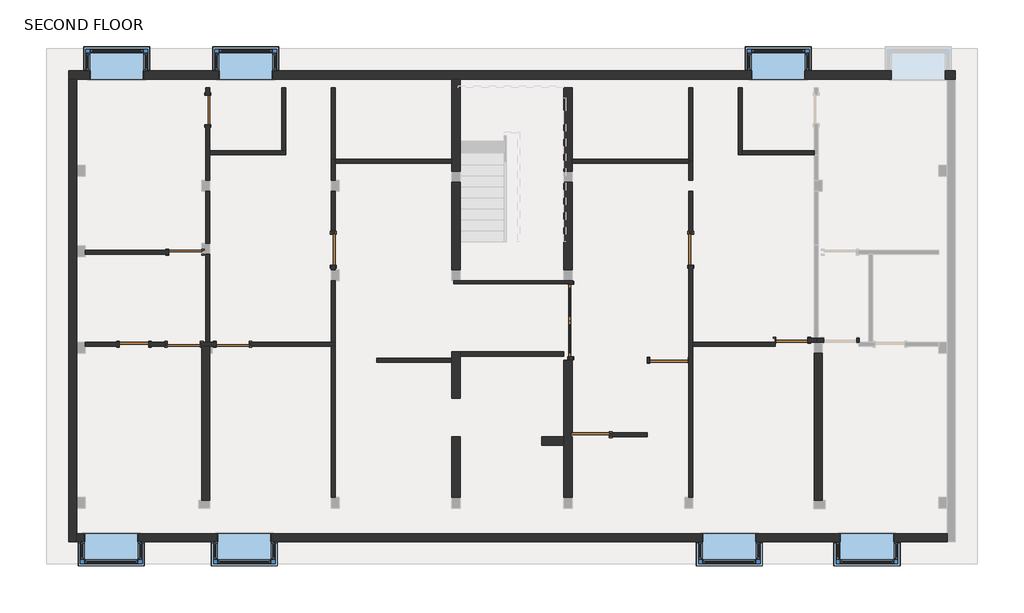
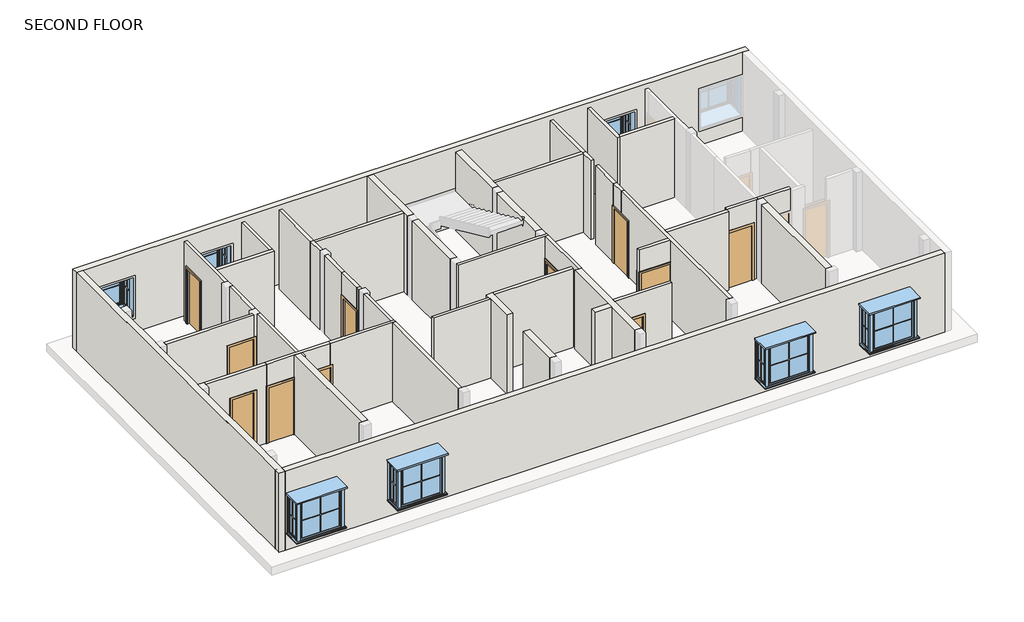
# One storey, part 1 of 2: 48 walls, 11 doors, 7 windows.
"""IFC4 building model written with IfcOpenShell, lengths in millimetres."""

from ifc_helpers import new_model, si_unit, frame, origin, place, context, project, spatial, polyline, outline, extrude, faceted_brep, transform, mapped, element, save
from components import door_04ab2522, m_door_single_panel_05506f71, door_07b5d71c, door_85b31ab1, door_1991e9a2, door_4c0a2014, door_82def9da, m_door_single_panel_3_x7_f8176753, m_door_single_panel_3_x7_ebb67e73, window_19bbd869

model = new_model("IFC4")

# Units and contexts
model_context = context("Model", 3, world=origin())
ifc_project = project(units=[si_unit("LENGTHUNIT", "METRE", prefix="MILLI")], contexts=[model_context])

# Site, building, storey
site = spatial("IfcSite", under=ifc_project)
building = spatial("IfcBuilding", under=site)
storey = spatial("IfcBuildingStorey", under=building, Name="SECOND FLOOR", Elevation=9601.2)

# Doors
placement = place(None, origin())
door_shape = door_04ab2522(model_context)
element("IfcDoor", 1, ObjectType="M_Door-Double-Glass : 6'7\"X7'", at=placement, inside=storey, context=model_context, shape_type="MappedRepresentation", body=[
    mapped(door_shape, transform((1217.5394962, 1183.3817656, 9601.2), x_axis=(0.0, 1.0, 0.0), y_axis=(-1.0, 0.0, 0.0), z_axis=(0.0, 0.0, 1.0))),
])
m_door_single_panel_shape = m_door_single_panel_05506f71(model_context)
element("IfcDoor", 2, ObjectType="M_Door-Single-Panel", at=placement, inside=storey, context=model_context, shape_type="MappedRepresentation", body=[
    mapped(m_door_single_panel_shape, transform((1745.3012085, -1975.7432663, 9601.2), x_axis=(-1.0, 0.0, 0.0), y_axis=(0.0, -1.0, 0.0), z_axis=(0.0, 0.0, 1.0))),
])
element("IfcDoor", 3, ObjectType="M_Door-Single-Panel", at=placement, inside=storey, context=model_context, shape_type="MappedRepresentation", body=[
    mapped(m_door_single_panel_shape, transform((3933.4813133, 90.9578621, 9601.2), x_axis=(1.0, 0.0, 0.0), y_axis=(0.0, 1.0, 0.0), z_axis=(0.0, 0.0, 1.0))),
])
door_2_shape = door_07b5d71c(model_context)
element("IfcDoor", 4, ObjectType="M_Door-Single-Panel : 2'10\"X7' 2", at=placement, inside=storey, context=model_context, shape_type="MappedRepresentation", body=[
    mapped(door_2_shape, transform((-5360.3487995, 3142.9626891, 9601.2), x_axis=(0.0, -1.0, 0.0), y_axis=(1.0, 0.0, 0.0), z_axis=(0.0, 0.0, 1.0))),
])
door_3_shape = door_85b31ab1(model_context)
element("IfcDoor", 5, ObjectType="M_Door-Single-Panel : 2'10\"X7' 2", at=placement, inside=storey, context=model_context, shape_type="MappedRepresentation", body=[
    mapped(door_3_shape, transform((4532.9512082, 3142.9626891, 9601.2), x_axis=(0.0, -1.0, 0.0), y_axis=(1.0, 0.0, 0.0), z_axis=(0.0, 0.0, 1.0))),
])
door_4_shape = door_1991e9a2(model_context)
element("IfcDoor", 6, ObjectType="M_Door-Single-Panel : 2'11\"X7' 3", at=placement, inside=storey, context=model_context, shape_type="MappedRepresentation", body=[
    mapped(door_4_shape, transform((7330.1405552, 640.4567334, 9601.2), x_axis=(1.0, 0.0, 0.0), y_axis=(0.0, 1.0, 0.0), z_axis=(0.0, 0.0, 1.0))),
])
door_5_shape = door_4c0a2014(model_context)
element("IfcDoor", 7, ObjectType="M_Door-Single-Panel : 2'8\"X7'", at=placement, inside=storey, context=model_context, shape_type="MappedRepresentation", body=[
    mapped(door_5_shape, transform((-10873.4462614, 526.1567334, 9601.2), x_axis=(1.0, 0.0, 0.0), y_axis=(0.0, 1.0, 0.0), z_axis=(0.0, 0.0, 1.0))),
])
door_6_shape = door_82def9da(model_context)
element("IfcDoor", 8, ObjectType="M_Door-Single-Panel : 2'8\"X7'", at=placement, inside=storey, context=model_context, shape_type="MappedRepresentation", body=[
    mapped(door_6_shape, transform((-8827.4487992, 7008.6751452, 9601.2), x_axis=(0.0, 1.0, 0.0), y_axis=(-1.0, 0.0, 0.0), z_axis=(0.0, 0.0, 1.0))),
])
m_door_single_panel_3_x7_shape = m_door_single_panel_3_x7_f8176753(model_context)
element("IfcDoor", 9, ObjectType="M_Door-Single-Panel : 3'X7'", at=placement, inside=storey, context=model_context, shape_type="MappedRepresentation", body=[
    mapped(m_door_single_panel_3_x7_shape, transform((-9456.0987989, 3078.8567332, 9601.2), x_axis=(1.0, 0.0, 0.0), y_axis=(0.0, 1.0, 0.0), z_axis=(0.0, 0.0, 1.0))),
])
element("IfcDoor", 10, ObjectType="M_Door-Single-Panel : 3'X7'", at=placement, inside=storey, context=model_context, shape_type="MappedRepresentation", body=[
    mapped(m_door_single_panel_3_x7_shape, transform((-8144.8381465, 526.1567334, 9601.2), x_axis=(-1.0, 0.0, 0.0), y_axis=(0.0, -1.0, 0.0), z_axis=(0.0, 0.0, 1.0))),
])
m_door_single_panel_3_x7_2_shape = m_door_single_panel_3_x7_ebb67e73(model_context)
element("IfcDoor", 11, ObjectType="M_Door-Single-Panel : 3'X7'", at=placement, inside=storey, context=model_context, shape_type="MappedRepresentation", body=[
    mapped(m_door_single_panel_3_x7_2_shape, transform((-9494.1987992, 526.1567334, 9601.2), x_axis=(1.0, 0.0, 0.0), y_axis=(0.0, 1.0, 0.0), z_axis=(0.0, 0.0, 1.0))),
])

# Walls
element("IfcWall", 12, ObjectType="3.5\"", at=placement, inside=storey, context=model_context, shape_type="Brep", body=[
    faceted_brep([(-2020.2487998, 2196.2067742, 9601.2), (1158.0082462, 2196.2067742, 9601.2), (1272.3082462, 2196.2067742, 9601.2), (1272.3082462, 2196.2067742, 12649.2), (1158.0082462, 2196.2067742, 12649.2), (-2020.2487998, 2196.2067742, 12649.2), (-2020.2487998, 2285.1067742, 9601.2), (-2020.2487998, 2285.1067742, 12649.2), (-1845.5417538, 2285.1067742, 12649.2), (1024.6582462, 2285.1067742, 12649.2), (1253.2582462, 2285.1067742, 12649.2), (1272.3082462, 2285.1067742, 12649.2), (1272.3082462, 2285.1067742, 9601.2), (1253.2582462, 2285.1067742, 9601.2), (1024.6582462, 2285.1067742, 9601.2), (-1845.5417538, 2285.1067742, 9601.2)], [[[0, 1, 2, 3, 4, 5]], [[6, 7, 8, 9, 10, 11, 12, 13, 14, 15]], [[2, 1, 0, 6, 15, 14, 13, 12]], [[5, 4, 3, 11, 10, 9, 8, 7]], [[0, 5, 7, 6]], [[3, 2, 12, 11]]]),
])
element("IfcWall", 13, ObjectType="4.5\"", at=placement, inside=storey, context=model_context, shape_type="SweptSolid", body=[
    extrude(outline(polyline([(3132.0737955, 12649.2), (3628.3344162, 12649.2), (3628.3344162, 9601.2), (3574.7626891, 9601.2), (3574.7626891, 11734.8), (3132.0737955, 11734.8), (3132.0737955, 12649.2)])), frame((4475.8012082, 0.0, 0.0), z_axis=(1.0, 0.0, 0.0), x_axis=(0.0, 1.0, 0.0)), (0.0, 0.0, 1.0), 114.3),
])
element("IfcWall", 14, ObjectType="4.5\"", at=placement, inside=storey, context=model_context, shape_type="SweptSolid", body=[
    extrude(outline(polyline([(2711.1626891, 12649.2), (3671.8272228, 12649.2), (3671.8272228, 9601.2), (3574.7626891, 9601.2), (3574.7626891, 11734.8), (2711.1626891, 11734.8), (2711.1626891, 12649.2)])), frame((-5417.4987995, 0.0, 0.0), z_axis=(1.0, 0.0, 0.0), x_axis=(0.0, 1.0, 0.0)), (0.0, 0.0, 1.0), 114.3),
])
element("IfcWall", 15, ObjectType="4.5\"", at=placement, inside=storey, context=model_context, shape_type="Brep", body=[
    faceted_brep([(-7690.1644155, 469.0067334, 12649.2), (-8713.148796, 469.0067334, 12649.2), (-8771.750543, 469.0067334, 12649.2), (-9000.350543, 469.0067334, 12649.2), (-10009.8462614, 469.0067334, 12649.2), (-10009.8462614, 469.0067334, 9601.2), (-9951.3987992, 469.0067334, 9601.2), (-9951.3987992, 469.0067334, 11734.8), (-9036.9987992, 469.0067334, 11734.8), (-9036.9987992, 469.0067334, 9601.2), (-9000.350543, 469.0067334, 9601.2), (-8771.750543, 469.0067334, 9601.2), (-8713.148796, 469.0067334, 9601.2), (-8602.0381465, 469.0067334, 9601.2), (-8602.0381465, 469.0067334, 11734.8), (-7690.1644155, 469.0067334, 11734.8), (-10009.8462614, 583.3067334, 12649.2), (-7690.1644155, 583.3067334, 12649.2), (-7690.1644155, 583.3067334, 11734.8), (-8602.0381465, 583.3067334, 11734.8), (-8602.0381465, 583.3067334, 9601.2), (-9036.9987992, 583.3067334, 9601.2), (-9036.9987992, 583.3067334, 11734.8), (-9951.3987992, 583.3067334, 11734.8), (-9951.3987992, 583.3067334, 9601.2), (-10009.8462614, 583.3067334, 9601.2)], [[[0, 1, 2, 3, 4, 5, 6, 7, 8, 9, 10, 11, 12, 13, 14, 15]], [[16, 17, 18, 19, 20, 21, 22, 23, 24, 25]], [[5, 25, 24, 6]], [[9, 21, 20, 13, 12, 11, 10]], [[17, 0, 15, 18]], [[4, 3, 2, 1, 0, 17, 16]], [[5, 4, 16, 25]], [[8, 22, 21, 9]], [[7, 23, 22, 8]], [[23, 7, 6, 24]], [[19, 14, 13, 20]], [[14, 19, 18, 15]]]),
])
element("IfcWall", 16, ObjectType="4.5\"", at=placement, inside=storey, context=model_context, shape_type="Brep", body=[
    faceted_brep([(8000.0512079, 583.3067334, 9601.2), (8000.0512079, 583.3067334, 12649.2), (7942.9012047, 583.3067334, 12649.2), (6862.7668241, 583.3067334, 12649.2), (6862.7668241, 583.3067334, 9601.2), (6885.6405552, 583.3067334, 9601.2), (6885.6405552, 583.3067334, 11734.8), (7774.6405552, 583.3067334, 11734.8), (7774.6405552, 583.3067334, 9601.2), (7942.9012047, 583.3067334, 9601.2), (8000.0512079, 697.6067334, 12649.2), (8000.0512079, 697.6067334, 9601.2), (7942.9012079, 697.6067334, 9601.2), (7774.6405552, 697.6067334, 9601.2), (7774.6405552, 697.6067334, 11734.8), (6885.6405552, 697.6067334, 11734.8), (6885.6405552, 697.6067334, 9601.2), (6862.7668241, 697.6067334, 9601.2), (6862.7668241, 697.6067334, 12649.2), (7942.9012079, 697.6067334, 12649.2)], [[[0, 1, 2, 3, 4, 5, 6, 7, 8, 9]], [[10, 11, 12, 13, 14, 15, 16, 17, 18, 19]], [[4, 17, 16, 5]], [[11, 0, 9, 8, 13, 12]], [[1, 0, 11, 10]], [[3, 2, 1, 10, 19, 18]], [[4, 3, 18, 17]], [[7, 14, 13, 8]], [[14, 7, 6, 15]], [[15, 6, 5, 16]]]),
])
element("IfcWall", 17, ObjectType="4.5\"", at=placement, inside=storey, context=model_context, shape_type="Brep", body=[
    faceted_brep([(9187.5012047, 583.3067334, 9601.2), (9187.5012047, 583.3067334, 12649.2), (8171.5012047, 583.3067334, 12649.2), (8000.0512079, 583.3067334, 12649.2), (8000.0512079, 583.3067334, 9601.2), (8171.5012047, 583.3067334, 9601.2), (8209.6012079, 583.3067334, 9601.2), (8209.6012079, 583.3067334, 11734.8), (9124.0012079, 583.3067334, 11734.8), (9124.0012079, 583.3067334, 9601.2), (9187.5012047, 697.6067334, 12649.2), (9187.5012047, 697.6067334, 9601.2), (9124.0012079, 697.6067334, 9601.2), (9124.0012079, 697.6067334, 11734.8), (8209.6012079, 697.6067334, 11734.8), (8209.6012079, 697.6067334, 9601.2), (8057.2012079, 697.6067334, 9601.2), (8000.0512079, 697.6067334, 9601.2), (8000.0512079, 697.6067334, 12649.2), (8057.2012079, 697.6067334, 12649.2)], [[[0, 1, 2, 3, 4, 5, 6, 7, 8, 9]], [[10, 11, 12, 13, 14, 15, 16, 17, 18, 19]], [[11, 0, 9, 12]], [[4, 17, 16, 15, 6, 5]], [[1, 0, 11, 10]], [[3, 2, 1, 10, 19, 18]], [[4, 3, 18, 17]], [[7, 14, 13, 8]], [[8, 13, 12, 9]], [[14, 7, 6, 15]]]),
])
element("IfcWall", 18, ObjectType="4.5\"", at=placement, inside=storey, context=model_context, shape_type="SweptSolid", body=[
    extrude(outline(polyline([(9601.2, 3334.0114184), (12649.2, 3334.0114184), (12649.2, 1250.0012085), (11734.8, 1250.0012085), (11734.8, 2278.7012085), (9601.2, 2278.7012085), (9601.2, 3334.0114184)])), frame((0.0, -2032.8932663, 0.0), z_axis=(0.0, 1.0, 0.0), x_axis=(0.0, 0.0, 1.0)), (0.0, 0.0, 1.0), 114.3),
])
element("IfcWall", 19, ObjectType="4.5\"", at=placement, inside=storey, context=model_context, shape_type="SweptSolid", body=[
    extrude(outline(polyline([(11734.8, 4466.8813133), (9601.2, 4466.8813133), (9601.2, 4475.8012082), (12649.2, 4475.8012082), (12649.2, 3334.0114184), (9601.2, 3334.0114184), (9601.2, 3400.0813133), (11734.8, 3400.0813133), (11734.8, 4466.8813133)])), frame((0.0, 33.8078621, 0.0), z_axis=(0.0, 1.0, 0.0), x_axis=(0.0, 0.0, 1.0)), (0.0, 0.0, 1.0), 114.3),
])
element("IfcWall", 20, ObjectType="4.5\"", at=placement, inside=storey, context=model_context, shape_type="SweptSolid", body=[
    extrude(outline(polyline([(1021.4012085, 202.3067742), (-1848.7987998, 202.3067742), (-1848.7987998, 316.6067742), (1021.4012085, 316.6067742), (1021.4012085, 202.3067742)])), frame((0.0, 0.0, 9601.2), z_axis=(0.0, 0.0, 1.0), x_axis=(1.0, 0.0, 0.0)), (0.0, 0.0, 1.0), 3048.0),
])
element("IfcWall", 21, ObjectType="4.5\"", at=placement, inside=storey, context=model_context, shape_type="Brep", body=[
    faceted_brep([(1158.0082462, 2196.2067742, 9601.2), (1158.0082462, 2186.6817656, 9601.2), (1158.0082462, 2186.6817656, 11734.8), (1158.0082462, 180.0817656, 11734.8), (1158.0082462, 180.0817656, 9601.2), (1158.0082462, 90.9578621, 9601.2), (1158.0082462, 90.9578621, 12649.2), (1158.0082462, 2196.2067742, 12649.2), (1272.3082462, 2186.6817656, 11734.8), (1272.3082462, 2186.6817656, 9601.2), (1272.3082462, 2196.2067742, 9601.2), (1272.3082462, 2196.2067742, 12649.2), (1272.3082462, 90.9578621, 12649.2), (1272.3082462, 90.9578621, 9601.2), (1272.3082462, 180.0817656, 9601.2), (1272.3082462, 180.0817656, 11734.8), (1250.0012085, 90.9578621, 9601.2), (1250.0012085, 90.9578621, 12649.2)], [[[0, 1, 2, 3, 4, 5, 6, 7]], [[8, 9, 10, 11, 12, 13, 14, 15]], [[14, 13, 16, 5, 4]], [[10, 9, 1, 0]], [[6, 5, 16, 13, 12, 17]], [[7, 6, 17, 12, 11]], [[0, 7, 11, 10]], [[2, 1, 9, 8]], [[3, 2, 8, 15]], [[4, 3, 15, 14]]]),
])
element("IfcWall", 22, ObjectType="4.5\"", at=placement, inside=storey, context=model_context, shape_type="Brep", body=[
    faceted_brep([(1250.0012085, 5536.3067329, 9601.2), (4475.8012082, 5536.3067329, 9601.2), (4475.8012082, 5536.3067329, 12649.2), (1250.0012085, 5536.3067329, 12649.2), (1250.0012085, 5650.6067329, 9601.2), (1250.0012085, 5650.6067329, 12649.2), (4475.8012082, 5650.6067329, 12649.2), (4475.8012082, 5650.6067329, 9601.2), (4475.8012082, 5593.4567329, 9601.2), (4475.8012082, 5593.4567329, 12649.2)], [[[0, 1, 2, 3]], [[4, 5, 6, 7]], [[1, 0, 4, 7, 8]], [[3, 2, 9, 6, 5]], [[2, 1, 8, 7, 6, 9]], [[0, 3, 5, 4]]]),
])
element("IfcWall", 23, ObjectType="4.5\"", at=placement, inside=storey, context=model_context, shape_type="SweptSolid", body=[
    extrude(outline(polyline([(-5417.4987995, -3709.2932193), (-5417.4987995, 469.0067334), (-5303.1987995, 469.0067334), (-5303.1987995, -3709.2932193), (-5417.4987995, -3709.2932193)])), frame((0.0, 0.0, 9601.2), z_axis=(0.0, 0.0, 1.0), x_axis=(1.0, 0.0, 0.0)), (0.0, 0.0, 1.0), 3048.0),
])
element("IfcWall", 24, ObjectType="4.5\" 2", at=placement, inside=storey, context=model_context, shape_type="SweptSolid", body=[
    extrude(outline(polyline([(12649.2, -8998.8987989), (12649.2, -12224.6987989), (9601.2, -12224.6987989), (9601.2, -9913.2987989), (11734.8, -9913.2987989), (11734.8, -8998.8987989), (12649.2, -8998.8987989)])), frame((0.0, 3021.7067332, 0.0), z_axis=(0.0, 1.0, 0.0), x_axis=(0.0, 0.0, 1.0)), (0.0, 0.0, 1.0), 114.3),
])
element("IfcWall", 25, ObjectType="4.5\" 2", at=placement, inside=storey, context=model_context, shape_type="SweptSolid", body=[
    extrude(outline(polyline([(-8770.2987992, 4761.606733), (-8770.2987992, 3326.5067332), (-8884.5987992, 3326.5067332), (-8884.5987992, 4761.606733), (-8770.2987992, 4761.606733)])), frame((0.0, 0.0, 9601.2), z_axis=(0.0, 0.0, 1.0), x_axis=(1.0, 0.0, 0.0)), (0.0, 0.0, 1.0), 3048.0),
])
element("IfcWall", 26, ObjectType="4.5\" 2", at=placement, inside=storey, context=model_context, shape_type="Brep", body=[
    faceted_brep([(-8770.2987992, 7415.0751452, 11734.8), (-8770.2987992, 7415.0751452, 9601.2), (-8770.2987992, 7631.8067329, 9601.2), (-8770.2987992, 7631.8067329, 12649.2), (-8770.2987992, 5879.2067329, 12649.2), (-8770.2987992, 5764.9067329, 12649.2), (-8770.2987992, 5066.406733, 12649.2), (-8770.2987992, 5066.406733, 9601.2), (-8770.2987992, 5764.9067329, 9601.2), (-8770.2987992, 5879.2067329, 9601.2), (-8770.2987992, 6602.2751452, 9601.2), (-8770.2987992, 6602.2751452, 11734.8), (-8884.5987992, 7631.8067329, 9601.2), (-8884.5987992, 7415.0751452, 9601.2), (-8884.5987992, 7415.0751452, 11734.8), (-8884.5987992, 6602.2751452, 11734.8), (-8884.5987992, 6602.2751452, 9601.2), (-8884.5987992, 5066.406733, 9601.2), (-8884.5987992, 5066.406733, 12649.2), (-8884.5987992, 7631.8067329, 12649.2)], [[[0, 1, 2, 3, 4, 5, 6, 7, 8, 9, 10, 11]], [[12, 13, 14, 15, 16, 17, 18, 19]], [[2, 1, 13, 12]], [[10, 9, 8, 7, 17, 16]], [[3, 2, 12, 19]], [[6, 5, 4, 3, 19, 18]], [[7, 6, 18, 17]], [[14, 13, 1, 0]], [[15, 14, 0, 11]], [[16, 15, 11, 10]]]),
])
element("IfcWall", 27, ObjectType="4.5\" 2", at=placement, inside=storey, context=model_context, shape_type="Brep", body=[
    faceted_brep([(-8770.2987992, 5764.9067329, 9601.2), (-6674.7987994, 5764.9067329, 9601.2), (-6674.7987994, 5764.9067329, 12649.2), (-8770.2987992, 5764.9067329, 12649.2), (-8770.2987992, 5879.2067329, 9601.2), (-8770.2987992, 5879.2067329, 12649.2), (-6789.0987994, 5879.2067329, 12649.2), (-6674.7987994, 5879.2067329, 12649.2), (-6674.7987994, 5879.2067329, 9601.2), (-6789.0987994, 5879.2067329, 9601.2)], [[[0, 1, 2, 3]], [[4, 5, 6, 7, 8, 9]], [[1, 0, 4, 9, 8]], [[3, 2, 7, 6, 5]], [[0, 3, 5, 4]], [[2, 1, 8, 7]]]),
])
element("IfcWall", 28, ObjectType="4.5\" 2", at=placement, inside=storey, context=model_context, shape_type="SweptSolid", body=[
    extrude(outline(polyline([(-6674.7987994, 7631.8067329), (-6674.7987994, 5879.2067329), (-6789.0987994, 5879.2067329), (-6789.0987994, 7631.8067329), (-6674.7987994, 7631.8067329)])), frame((0.0, 0.0, 9601.2), z_axis=(0.0, 0.0, 1.0), x_axis=(1.0, 0.0, 0.0)), (0.0, 0.0, 1.0), 3048.0),
])
element("IfcWall", 29, ObjectType="4.5\" 2", at=placement, inside=storey, context=model_context, shape_type="SweptSolid", body=[
    extrude(outline(polyline([(11734.8, -10467.0462614), (9601.2, -10467.0462614), (9601.2, -10009.8462614), (12649.2, -10009.8462614), (12649.2, -12224.6987989), (9601.2, -12224.6987989), (9601.2, -11279.8462614), (11734.8, -11279.8462614), (11734.8, -10467.0462614)])), frame((0.0, 469.0067334, 0.0), z_axis=(0.0, 1.0, 0.0), x_axis=(0.0, 0.0, 1.0)), (0.0, 0.0, 1.0), 114.3),
])
element("IfcWall", 30, ObjectType="4.5\" 2", at=placement, inside=storey, context=model_context, shape_type="SweptSolid", body=[
    extrude(outline(polyline([(-8770.298796, 3021.7067332), (-8770.298796, 583.3067804), (-8884.598796, 583.3067804), (-8884.598796, 3021.7067332), (-8770.298796, 3021.7067332)])), frame((0.0, 0.0, 9601.2), z_axis=(0.0, 0.0, 1.0), x_axis=(1.0, 0.0, 0.0)), (0.0, 0.0, 1.0), 3048.0),
])
element("IfcWall", 31, ObjectType="4.5\" 2", at=placement, inside=storey, context=model_context, shape_type="Brep", body=[
    faceted_brep([(-5303.1987995, 469.0067334, 12649.2), (-5417.4987995, 469.0067334, 12649.2), (-7690.1644155, 469.0067334, 12649.2), (-7690.1644155, 469.0067334, 11734.8), (-7687.6381465, 469.0067334, 11734.8), (-7687.6381465, 469.0067334, 9601.2), (-5417.4987995, 469.0067334, 9601.2), (-5303.1987995, 469.0067334, 9601.2), (-7690.1644155, 583.3067334, 12649.2), (-5417.4987995, 583.3067334, 12649.2), (-5303.1987995, 583.3067334, 12649.2), (-5303.1987995, 583.3067334, 9601.2), (-5417.4987995, 583.3067334, 9601.2), (-7687.6381465, 583.3067334, 9601.2), (-7687.6381465, 583.3067334, 11734.8), (-7690.1644155, 583.3067334, 11734.8)], [[[0, 1, 2, 3, 4, 5, 6, 7]], [[8, 9, 10, 11, 12, 13, 14, 15]], [[11, 7, 6, 5, 13, 12]], [[2, 1, 0, 10, 9, 8]], [[2, 8, 15, 3]], [[0, 7, 11, 10]], [[14, 4, 3, 15]], [[4, 14, 13, 5]]]),
])
element("IfcWall", 32, ObjectType="4.5\" 2", at=placement, inside=storey, context=model_context, shape_type="SweptSolid", body=[
    extrude(outline(polyline([(-5303.1987995, 2285.1067802), (-5303.1987995, 583.3067334), (-5417.4987995, 583.3067334), (-5417.4987995, 2285.1067802), (-5303.1987995, 2285.1067802)])), frame((0.0, 0.0, 9601.2), z_axis=(0.0, 0.0, 1.0), x_axis=(1.0, 0.0, 0.0)), (0.0, 0.0, 1.0), 3048.0),
])
element("IfcWall", 33, ObjectType="4.5\" 2", at=placement, inside=storey, context=model_context, shape_type="Brep", body=[
    faceted_brep([(-5303.1987995, 2589.9067802, 9601.2), (-5303.1987995, 2711.1626891, 9601.2), (-5303.1987995, 2711.1626891, 11734.8), (-5303.1987995, 2711.1626891, 12649.2), (-5303.1987995, 2589.9067802, 12649.2), (-5417.4987995, 2589.9067802, 9601.2), (-5417.4987995, 2589.9067802, 12649.2), (-5417.4987995, 2711.1626891, 12649.2), (-5417.4987995, 2711.1626891, 11734.8), (-5417.4987995, 2711.1626891, 9601.2)], [[[0, 1, 2, 3, 4]], [[5, 6, 7, 8, 9]], [[1, 0, 5, 9]], [[3, 2, 1, 9, 8, 7]], [[4, 3, 7, 6]], [[0, 4, 6, 5]]]),
])
element("IfcWall", 34, ObjectType="4.5\" 2", at=placement, inside=storey, context=model_context, shape_type="SweptSolid", body=[
    extrude(outline(polyline([(-5303.1987995, 4761.606733), (-5303.1987995, 3671.8272228), (-5417.4987995, 3671.8272228), (-5417.4987995, 4761.606733), (-5303.1987995, 4761.606733)])), frame((0.0, 0.0, 9601.2), z_axis=(0.0, 0.0, 1.0), x_axis=(1.0, 0.0, 0.0)), (0.0, 0.0, 1.0), 3048.0),
])
element("IfcWall", 35, ObjectType="4.5\" 2", at=placement, inside=storey, context=model_context, shape_type="Brep", body=[
    faceted_brep([(-5303.1987995, 5066.406733, 9601.2), (-5303.1987995, 5536.3067329, 9601.2), (-5303.1987995, 5650.6067329, 9601.2), (-5303.1987995, 5650.6067329, 12649.2), (-5303.1987995, 5536.3067329, 12649.2), (-5303.1987995, 5066.406733, 12649.2), (-5417.4987995, 5066.406733, 9601.2), (-5417.4987995, 5066.406733, 12649.2), (-5417.4987995, 5650.6067329, 12649.2), (-5417.4987995, 5650.6067329, 9601.2)], [[[0, 1, 2, 3, 4, 5]], [[6, 7, 8, 9]], [[2, 1, 0, 6, 9]], [[5, 4, 3, 8, 7]], [[0, 5, 7, 6]], [[3, 2, 9, 8]]]),
])
element("IfcWall", 36, ObjectType="4.5\" 2", at=placement, inside=storey, context=model_context, shape_type="SweptSolid", body=[
    extrude(outline(polyline([(-2077.3987998, 5536.3067329), (-5303.1987995, 5536.3067329), (-5303.1987995, 5650.6067329), (-2077.3987998, 5650.6067329), (-2077.3987998, 5536.3067329)])), frame((0.0, 0.0, 9601.2), z_axis=(0.0, 0.0, 1.0), x_axis=(1.0, 0.0, 0.0)), (0.0, 0.0, 1.0), 3048.0),
])
element("IfcWall", 37, ObjectType="4.5\" 2", at=placement, inside=storey, context=model_context, shape_type="SweptSolid", body=[
    extrude(outline(polyline([(-5417.4987995, 5650.6067329), (-5417.4987995, 7631.8067329), (-5303.1987995, 7631.8067329), (-5303.1987995, 5650.6067329), (-5417.4987995, 5650.6067329)])), frame((0.0, 0.0, 9601.2), z_axis=(0.0, 0.0, 1.0), x_axis=(1.0, 0.0, 0.0)), (0.0, 0.0, 1.0), 3048.0),
])
element("IfcWall", 38, ObjectType="4.5\" 2", at=placement, inside=storey, context=model_context, shape_type="Brep", body=[
    faceted_brep([(4475.8012082, 5593.4567329, 9601.2), (4475.8012082, 5536.3067329, 9601.2), (4475.8012082, 5066.40678, 9601.2), (4475.8012082, 5066.40678, 12649.2), (4475.8012082, 5536.3067329, 12649.2), (4475.8012082, 5593.4567329, 12649.2), (4590.1012082, 5593.4567329, 9601.2), (4590.1012082, 5593.4567329, 12649.2), (4590.1012082, 5066.40678, 12649.2), (4590.1012082, 5066.40678, 9601.2)], [[[0, 1, 2, 3, 4, 5]], [[6, 7, 8, 9]], [[2, 1, 0, 6, 9]], [[3, 2, 9, 8]], [[5, 4, 3, 8, 7]], [[0, 5, 7, 6]]]),
])
element("IfcWall", 39, ObjectType="4.5\" 2", at=placement, inside=storey, context=model_context, shape_type="SweptSolid", body=[
    extrude(outline(polyline([(4475.8012082, 3628.3344162), (4475.8012082, 4761.606733), (4590.1012082, 4761.606733), (4590.1012082, 3628.3344162), (4475.8012082, 3628.3344162)])), frame((0.0, 0.0, 9601.2), z_axis=(0.0, 0.0, 1.0), x_axis=(1.0, 0.0, 0.0)), (0.0, 0.0, 1.0), 3048.0),
])
element("IfcWall", 40, ObjectType="4.5\" 2", at=placement, inside=storey, context=model_context, shape_type="Brep", body=[
    faceted_brep([(4475.8012082, -3709.2932193, 9601.2), (4475.8012082, -3709.2932193, 12649.2), (4475.8012082, 33.8078621, 12649.2), (4475.8012082, 148.1078621, 12649.2), (4475.8012082, 3132.0737955, 12649.2), (4475.8012082, 3132.0737955, 11734.8), (4475.8012082, 2711.1626891, 11734.8), (4475.8012082, 2711.1626891, 9601.2), (4475.8012082, 148.1078621, 9601.2), (4475.8012082, 33.8078621, 9601.2), (4590.1012082, -3709.2932193, 12649.2), (4590.1012082, -3709.2932193, 9601.2), (4590.1012082, 469.0067334, 9601.2), (4590.1012082, 583.3067334, 9601.2), (4590.1012082, 2711.1626891, 9601.2), (4590.1012082, 2711.1626891, 11734.8), (4590.1012082, 3132.0737955, 11734.8), (4590.1012082, 3132.0737955, 12649.2), (4590.1012082, 583.3067334, 12649.2), (4590.1012082, 469.0067334, 12649.2)], [[[0, 1, 2, 3, 4, 5, 6, 7, 8, 9]], [[10, 11, 12, 13, 14, 15, 16, 17, 18, 19]], [[11, 0, 9, 8, 7, 14, 13, 12]], [[1, 0, 11, 10]], [[4, 3, 2, 1, 10, 19, 18, 17]], [[4, 17, 16, 5]], [[6, 15, 14, 7]], [[15, 6, 5, 16]]]),
])
element("IfcWall", 41, ObjectType="4.5\" 2", at=placement, inside=storey, context=model_context, shape_type="SweptSolid", body=[
    extrude(outline(polyline([(6862.7668241, 469.0067334), (4590.1012082, 469.0067334), (4590.1012082, 583.3067334), (6862.7668241, 583.3067334), (6862.7668241, 469.0067334)])), frame((0.0, 0.0, 9601.2), z_axis=(0.0, 0.0, 1.0), x_axis=(1.0, 0.0, 0.0)), (0.0, 0.0, 1.0), 3048.0),
])
element("IfcWall", 42, ObjectType="4.5\" 2", at=placement, inside=storey, context=model_context, shape_type="Brep", body=[
    faceted_brep([(4590.1012082, 5593.4567329, 9601.2), (4590.1012082, 7631.8067329, 9601.2), (4590.1012082, 7631.8067329, 12649.2), (4590.1012082, 5593.4567329, 12649.2), (4475.8012082, 5593.4567329, 9601.2), (4475.8012082, 5593.4567329, 12649.2), (4475.8012082, 5650.6067329, 12649.2), (4475.8012082, 7631.8067329, 12649.2), (4475.8012082, 7631.8067329, 9601.2), (4475.8012082, 5650.6067329, 9601.2)], [[[0, 1, 2, 3]], [[4, 5, 6, 7, 8, 9]], [[1, 0, 4, 9, 8]], [[2, 1, 8, 7]], [[3, 2, 7, 6, 5]], [[0, 3, 5, 4]]]),
])
element("IfcWall", 43, ObjectType="4.5\" 2", at=placement, inside=storey, context=model_context, shape_type="Brep", body=[
    faceted_brep([(5847.401208, 7631.8067329, 9601.2), (5847.401208, 5764.9067329, 9601.2), (5847.401208, 5764.9067329, 12649.2), (5847.401208, 7631.8067329, 12649.2), (5961.701208, 7631.8067329, 9601.2), (5961.701208, 7631.8067329, 12649.2), (5961.701208, 5879.2067329, 12649.2), (5961.701208, 5764.9067329, 12649.2), (5961.701208, 5764.9067329, 9601.2), (5961.701208, 5879.2067329, 9601.2)], [[[0, 1, 2, 3]], [[4, 5, 6, 7, 8, 9]], [[1, 0, 4, 9, 8]], [[3, 2, 7, 6, 5]], [[0, 3, 5, 4]], [[2, 1, 8, 7]]]),
])
element("IfcWall", 44, ObjectType="4.5\" 2", at=placement, inside=storey, context=model_context, shape_type="SweptSolid", body=[
    extrude(outline(polyline([(7942.9012079, 5764.9067329), (5961.701208, 5764.9067329), (5961.701208, 5879.2067329), (7942.9012079, 5879.2067329), (7942.9012079, 5764.9067329)])), frame((0.0, 0.0, 9601.2), z_axis=(0.0, 0.0, 1.0), x_axis=(1.0, 0.0, 0.0)), (0.0, 0.0, 1.0), 3048.0),
])
element("IfcWall", 45, ObjectType="4.5\" 2", at=placement, inside=storey, context=model_context, shape_type="SweptSolid", body=[
    extrude(outline(polyline([(-2077.3987998, 33.8078621), (-4161.4090098, 33.8078621), (-4161.4090098, 148.1078621), (-2077.3987998, 148.1078621), (-2077.3987998, 33.8078621)])), frame((0.0, 0.0, 9601.2), z_axis=(0.0, 0.0, 1.0), x_axis=(1.0, 0.0, 0.0)), (0.0, 0.0, 1.0), 3048.0),
])
element("IfcWall", 46, ObjectType="9\"", at=placement, inside=storey, context=model_context, shape_type="Brep", body=[
    faceted_brep([(-12681.8987957, 7860.4067329, 9601.2), (-12453.2987957, 7860.4067329, 9601.2), (-2074.1417538, 7860.4067329, 9601.2), (-1845.5417538, 7860.4067329, 9601.2), (11625.9012075, 7860.4067329, 9601.2), (11854.5012075, 7860.4067329, 9601.2), (11854.5012075, 7860.4067329, 12649.2), (11625.9012075, 7860.4067329, 12649.2), (-1845.5417538, 7860.4067329, 12649.2), (-2074.1417538, 7860.4067329, 12649.2), (-12453.2987957, 7860.4067329, 12649.2), (-12681.8987957, 7860.4067329, 12649.2), (11575.8012075, 7860.4067329, 11752.0), (11575.8012075, 7860.4067329, 10201.2), (10075.8012075, 7860.4067329, 10201.2), (10075.8012075, 7860.4067329, 11752.0), (7702.301208, 7860.4067329, 11752.0), (7702.301208, 7860.4067329, 10201.2), (6202.301208, 7860.4067329, 10201.2), (6202.301208, 7860.4067329, 11752.0), (-7029.6987993, 7860.4067329, 11752.0), (-7029.6987993, 7860.4067329, 10201.2), (-8529.6987993, 7860.4067329, 10201.2), (-8529.6987993, 7860.4067329, 11752.0), (-10598.3987957, 7860.4067329, 11752.0), (-10598.3987957, 7860.4067329, 10201.2), (-12098.3987957, 7860.4067329, 10201.2), (-12098.3987957, 7860.4067329, 11752.0), (-12681.8987957, 8089.0067329, 9601.2), (-12681.8987957, 8089.0067329, 12649.2), (11854.5012075, 8089.0067329, 12649.2), (11854.5012075, 8089.0067329, 9601.2), (11575.8012075, 8089.0067329, 11752.0), (10075.8012075, 8089.0067329, 11752.0), (10075.8012075, 8089.0067329, 10201.2), (11575.8012075, 8089.0067329, 10201.2), (7702.301208, 8089.0067329, 11752.0), (6202.301208, 8089.0067329, 11752.0), (6202.301208, 8089.0067329, 10201.2), (7702.301208, 8089.0067329, 10201.2), (-7029.6987993, 8089.0067329, 11752.0), (-8529.6987993, 8089.0067329, 11752.0), (-8529.6987993, 8089.0067329, 10201.2), (-7029.6987993, 8089.0067329, 10201.2), (-10598.3987957, 8089.0067329, 11752.0), (-12098.3987957, 8089.0067329, 11752.0), (-12098.3987957, 8089.0067329, 10201.2), (-10598.3987957, 8089.0067329, 10201.2)], [[[0, 1, 2, 3, 4, 5, 6, 7, 8, 9, 10, 11], [12, 13, 14, 15], [16, 17, 18, 19], [20, 21, 22, 23], [24, 25, 26, 27]], [[28, 29, 30, 31], [32, 33, 34, 35], [36, 37, 38, 39], [40, 41, 42, 43], [44, 45, 46, 47]], [[5, 4, 3, 2, 1, 0, 28, 31]], [[11, 10, 9, 8, 7, 6, 30, 29]], [[6, 5, 31, 30]], [[0, 11, 29, 28]], [[13, 12, 32, 35]], [[14, 13, 35, 34]], [[15, 14, 34, 33]], [[12, 15, 33, 32]], [[17, 16, 36, 39]], [[18, 17, 39, 38]], [[19, 18, 38, 37]], [[16, 19, 37, 36]], [[21, 20, 40, 43]], [[22, 21, 43, 42]], [[23, 22, 42, 41]], [[20, 23, 41, 40]], [[25, 24, 44, 47]], [[26, 25, 47, 46]], [[27, 26, 46, 45]], [[24, 27, 45, 44]]]),
])
element("IfcWall", 47, ObjectType="9\"", at=placement, inside=storey, context=model_context, shape_type="Brep", body=[
    faceted_brep([(-12453.2987957, -4941.1932661, 9601.2), (-12453.2987957, -4712.5932661, 9601.2), (-12453.2987957, -4014.0932671, 9601.2), (-12453.2987957, -3709.2932671, 9601.2), (-12453.2987957, 278.5067334, 9601.2), (-12453.2987957, 583.3067334, 9601.2), (-12453.2987957, 2951.8567332, 9601.2), (-12453.2987957, 3256.6567332, 9601.2), (-12453.2987957, 5174.3567339, 9601.2), (-12453.2987957, 5479.1567339, 9601.2), (-12453.2987957, 7860.4067329, 9601.2), (-12453.2987957, 7860.4067329, 12649.2), (-12453.2987957, 5479.1567339, 12649.2), (-12453.2987957, 5174.3567339, 12649.2), (-12453.2987957, 3256.6567332, 12649.2), (-12453.2987957, 2951.8567332, 12649.2), (-12453.2987957, 583.3067334, 12649.2), (-12453.2987957, 278.5067334, 12649.2), (-12453.2987957, -3709.2932671, 12649.2), (-12453.2987957, -4014.0932671, 12649.2), (-12453.2987957, -4712.5932661, 12649.2), (-12453.2987957, -4941.1932661, 12649.2), (-12681.8987957, -4941.1932661, 9601.2), (-12681.8987957, -4941.1932661, 12649.2), (-12681.8987957, 7860.4067329, 12649.2), (-12681.8987957, 7860.4067329, 9601.2)], [[[0, 1, 2, 3, 4, 5, 6, 7, 8, 9, 10, 11, 12, 13, 14, 15, 16, 17, 18, 19, 20, 21]], [[22, 23, 24, 25]], [[10, 9, 8, 7, 6, 5, 4, 3, 2, 1, 0, 22, 25]], [[21, 20, 19, 18, 17, 16, 15, 14, 13, 12, 11, 24, 23]], [[11, 10, 25, 24]], [[0, 21, 23, 22]]]),
])
element("IfcWall", 48, ObjectType="9\"", at=placement, inside=storey, context=model_context, shape_type="Brep", body=[
    faceted_brep([(-12453.2987957, -4712.5932661, 9601.2), (-12453.2987957, -4014.0932671, 9601.2), (-12453.2987957, -3709.2932671, 9601.2), (-12453.2987957, 278.5067334, 9601.2), (-12453.2987957, 583.3067334, 9601.2), (-12453.2987957, 2951.8567332, 9601.2), (-12453.2987957, 3256.6567332, 9601.2), (-12453.2987957, 5174.3567339, 9601.2), (-12453.2987957, 5479.1567339, 9601.2), (-12453.2987957, 7860.4067329, 9601.2), (-12453.2987957, 7860.4067329, 12649.2), (-12453.2987957, 5479.1567339, 12649.2), (-12453.2987957, 5174.3567339, 12649.2), (-12453.2987957, 3256.6567332, 12649.2), (-12453.2987957, 2951.8567332, 12649.2), (-12453.2987957, 583.3067334, 12649.2), (-12453.2987957, 278.5067334, 12649.2), (-12453.2987957, -3709.2932671, 12649.2), (-12453.2987957, -4014.0932671, 12649.2), (-12453.2987957, -4712.5932661, 12649.2), (-12681.8987957, -4712.5932661, 9601.2), (-12681.8987957, -4712.5932661, 12649.2), (-12681.8987957, 7860.4067329, 12649.2), (-12681.8987957, 7860.4067329, 9601.2)], [[[0, 1, 2, 3, 4, 5, 6, 7, 8, 9, 10, 11, 12, 13, 14, 15, 16, 17, 18, 19]], [[20, 21, 22, 23]], [[9, 8, 7, 6, 5, 4, 3, 2, 1, 0, 20, 23]], [[19, 18, 17, 16, 15, 14, 13, 12, 11, 10, 22, 21]], [[10, 9, 23, 22]], [[0, 19, 21, 20]]]),
])
element("IfcWall", 49, ObjectType="9\"", at=placement, inside=storey, context=model_context, shape_type="Brep", body=[
    faceted_brep([(-9000.350543, 469.0067334, 9601.2), (-9000.350543, -3785.4932196, 9601.2), (-9000.350543, -3785.4932196, 12649.2), (-9000.350543, 469.0067334, 12649.2), (-8771.750543, 469.0067334, 9601.2), (-8771.750543, 469.0067334, 12649.2), (-8771.750543, 278.5067334, 12649.2), (-8771.750543, -3785.4932196, 12649.2), (-8771.750543, -3785.4932196, 9601.2), (-8771.750543, 278.5067334, 9601.2)], [[[0, 1, 2, 3]], [[4, 5, 6, 7, 8, 9]], [[1, 0, 4, 9, 8]], [[2, 1, 8, 7]], [[3, 2, 7, 6, 5]], [[0, 3, 5, 4]]]),
])
element("IfcWall", 50, ObjectType="9\"", at=placement, inside=storey, context=model_context, shape_type="Brep", body=[
    faceted_brep([(-2077.3987998, 316.6067742, 9601.2), (-2077.3987998, 148.1078621, 9601.2), (-2077.3987998, 33.8078621, 9601.2), (-2077.3987998, -972.2341552, 9601.2), (-2077.3987998, -972.2341552, 12649.2), (-2077.3987998, 33.8078621, 12649.2), (-2077.3987998, 148.1078621, 12649.2), (-2077.3987998, 316.6067742, 12649.2), (-1848.7987998, 316.6067742, 9601.2), (-1848.7987998, 316.6067742, 12649.2), (-1848.7987998, 202.3067742, 12649.2), (-1848.7987998, -972.2341552, 12649.2), (-1848.7987998, -972.2341552, 9601.2), (-1848.7987998, 202.3067742, 9601.2)], [[[0, 1, 2, 3, 4, 5, 6, 7]], [[8, 9, 10, 11, 12, 13]], [[3, 2, 1, 0, 8, 13, 12]], [[4, 3, 12, 11]], [[7, 6, 5, 4, 11, 10, 9]], [[0, 7, 9, 8]]]),
])
element("IfcWall", 51, ObjectType="9\"", at=placement, inside=storey, context=model_context, shape_type="SweptSolid", body=[
    extrude(outline(polyline([(-2077.3987998, -3709.2932663), (-2077.3987998, -2032.8932663), (-1848.7987998, -2032.8932663), (-1848.7987998, -3709.2932663), (-2077.3987998, -3709.2932663)])), frame((0.0, 0.0, 9601.2), z_axis=(0.0, 0.0, 1.0), x_axis=(1.0, 0.0, 0.0)), (0.0, 0.0, 1.0), 3048.0),
])
element("IfcWall", 52, ObjectType="9\"", at=placement, inside=storey, context=model_context, shape_type="SweptSolid", body=[
    extrude(outline(polyline([(1021.4012085, -2261.4932663), (412.152227, -2261.4932663), (412.152227, -2032.8932663), (1021.4012085, -2032.8932663), (1021.4012085, -2261.4932663)])), frame((0.0, 0.0, 9601.2), z_axis=(0.0, 0.0, 1.0), x_axis=(1.0, 0.0, 0.0)), (0.0, 0.0, 1.0), 3048.0),
])
element("IfcWall", 53, ObjectType="9\"", at=placement, inside=storey, context=model_context, shape_type="Brep", body=[
    faceted_brep([(1021.4012085, 90.9578621, 9601.2), (1021.4012085, -2032.8932663, 9601.2), (1021.4012085, -2261.4932663, 9601.2), (1021.4012085, -3709.2932193, 9601.2), (1021.4012085, -3709.2932193, 12649.2), (1021.4012085, -2261.4932663, 12649.2), (1021.4012085, -2032.8932663, 12649.2), (1021.4012085, 90.9578621, 12649.2), (1250.0012085, -3709.2932193, 12649.2), (1250.0012085, -3709.2932193, 9601.2), (1250.0012085, -2032.8932663, 9601.2), (1250.0012085, -2032.8932663, 11734.8), (1250.0012085, -1918.5932663, 11734.8), (1250.0012085, -1918.5932663, 9601.2), (1250.0012085, 90.9578621, 9601.2), (1250.0012085, 90.9578621, 12649.2), (1250.0012085, -1918.5932663, 12649.2), (1250.0012085, -2032.8932663, 12649.2), (1158.0082462, 90.9578621, 9601.2), (1211.9012085, -1918.5932663, 9601.2), (1211.9012085, -2032.8932663, 9601.2), (1158.0082462, 90.9578621, 12649.2), (1211.9012085, -1918.5932663, 11734.8), (1211.9012085, -2032.8932663, 11734.8)], [[[0, 1, 2, 3, 4, 5, 6, 7]], [[8, 9, 10, 11, 12, 13, 14, 15, 16, 17]], [[3, 2, 1, 0, 18, 14, 13, 19, 20, 10, 9]], [[4, 3, 9, 8]], [[7, 6, 5, 4, 8, 17, 16, 15, 21]], [[0, 7, 21, 15, 14, 18]], [[22, 19, 13, 12]], [[20, 23, 11, 10]], [[19, 22, 23, 20]], [[23, 22, 12, 11]]]),
])
element("IfcWall", 54, ObjectType="9\"", at=placement, inside=storey, context=model_context, shape_type="SweptSolid", body=[
    extrude(outline(polyline([(-2074.1417538, 5320.4067329), (-2074.1417538, 7860.4067329), (-1845.5417538, 7860.4067329), (-1845.5417538, 5320.4067329), (-2074.1417538, 5320.4067329)])), frame((0.0, 0.0, 9601.2), z_axis=(0.0, 0.0, 1.0), x_axis=(1.0, 0.0, 0.0)), (0.0, 0.0, 1.0), 3048.0),
])
element("IfcWall", 55, ObjectType="9\"", at=placement, inside=storey, context=model_context, shape_type="SweptSolid", body=[
    extrude(outline(polyline([(-2074.1417538, 2589.906774), (-2074.1417538, 5015.606774), (-1845.5417538, 5015.606774), (-1845.5417538, 2589.906774), (-2074.1417538, 2589.906774)])), frame((0.0, 0.0, 9601.2), z_axis=(0.0, 0.0, 1.0), x_axis=(1.0, 0.0, 0.0)), (0.0, 0.0, 1.0), 3048.0),
])
element("IfcWall", 56, ObjectType="9\"", at=placement, inside=storey, context=model_context, shape_type="Brep", body=[
    faceted_brep([(1021.4012085, 7631.8067329, 9601.2), (1021.4012085, 5320.4067329, 9601.2), (1021.4012085, 5320.4067329, 12649.2), (1021.4012085, 7631.8067329, 12649.2), (1250.0012085, 7631.8067329, 9601.2), (1250.0012085, 7631.8067329, 12649.2), (1250.0012085, 5650.6067329, 12649.2), (1250.0012085, 5536.3067329, 12649.2), (1250.0012085, 5320.4067329, 12649.2), (1250.0012085, 5320.4067329, 9601.2), (1250.0012085, 5536.3067329, 9601.2), (1250.0012085, 5650.6067329, 9601.2)], [[[0, 1, 2, 3]], [[4, 5, 6, 7, 8, 9, 10, 11]], [[1, 0, 4, 11, 10, 9]], [[2, 1, 9, 8]], [[3, 2, 8, 7, 6, 5]], [[0, 3, 5, 4]]]),
])
element("IfcWall", 57, ObjectType="9\"", at=placement, inside=storey, context=model_context, shape_type="Brep", body=[
    faceted_brep([(1021.4012085, 5015.6067329, 9601.2), (1021.4012085, 2589.9067742, 9601.2), (1021.4012085, 2589.9067742, 12649.2), (1021.4012085, 5015.6067329, 12649.2), (1250.0012085, 5015.6067329, 9601.2), (1250.0012085, 5015.6067329, 12649.2), (1250.0012085, 2589.9067742, 12649.2), (1250.0012085, 2589.9067742, 9601.2), (1024.6582462, 2589.9067742, 9601.2), (1024.6582462, 2589.9067742, 12649.2)], [[[0, 1, 2, 3]], [[4, 5, 6, 7]], [[1, 0, 4, 7, 8]], [[2, 1, 8, 7, 6, 9]], [[3, 2, 9, 6, 5]], [[0, 3, 5, 4]]]),
])
element("IfcWall", 58, ObjectType="9\"", at=placement, inside=storey, context=model_context, shape_type="SweptSolid", body=[
    extrude(outline(polyline([(7942.9012047, -3785.4932666), (7942.9012047, 278.5067334), (8171.5012047, 278.5067334), (8171.5012047, -3785.4932666), (7942.9012047, -3785.4932666)])), frame((0.0, 0.0, 9601.2), z_axis=(0.0, 0.0, 1.0), x_axis=(1.0, 0.0, 0.0)), (0.0, 0.0, 1.0), 3048.0),
])
element("IfcWall", 59, ObjectType="9\" 2", at=placement, inside=storey, context=model_context, shape_type="SweptSolid", body=[
    extrude(outline(polyline([(9601.2, -12453.2987957), (9601.2, 11625.9012075), (12649.2, 11625.9012075), (12649.2, -12453.2987957), (9601.2, -12453.2987957)]), holes=[polyline([(11752.0, 8658.6146942), (11752.0, 10158.6146942), (10201.2, 10158.6146942), (10201.2, 8658.6146942), (11752.0, 8658.6146942)]), polyline([(11752.0, 4849.7512082), (11752.0, 6349.7512082), (10201.2, 6349.7512082), (10201.2, 4849.7512082), (11752.0, 4849.7512082)]), polyline([(11752.0, -8569.250543), (11752.0, -7069.250543), (10201.2, -7069.250543), (10201.2, -8569.250543), (11752.0, -8569.250543)]), polyline([(11752.0, -12250.7987957), (11752.0, -10750.7987957), (10201.2, -10750.7987957), (10201.2, -12250.7987957), (11752.0, -12250.7987957)])]), frame((0.0, -4941.1932661, 0.0), z_axis=(0.0, 1.0, 0.0), x_axis=(0.0, 0.0, 1.0)), (0.0, 0.0, 1.0), 228.6),
])

# Windows
window_shape = window_19bbd869(model_context)
element("IfcWindow", 60, ObjectType="4'.8\"x3'.8\"", at=placement, inside=storey, context=model_context, shape_type="MappedRepresentation", body=[
    mapped(window_shape, transform((-11500.7987957, -4826.8932661, 9601.2), x_axis=(-1.0, 0.0, 0.0), y_axis=(0.0, -1.0, 0.0), z_axis=(0.0, 0.0, 1.0))),
])
element("IfcWindow", 61, ObjectType="4'.8\"x3'.8\"", at=placement, inside=storey, context=model_context, shape_type="MappedRepresentation", body=[
    mapped(window_shape, transform((-7819.250543, -4826.8932661, 9601.2), x_axis=(-1.0, 0.0, 0.0), y_axis=(0.0, -1.0, 0.0), z_axis=(0.0, 0.0, 1.0))),
])
element("IfcWindow", 62, ObjectType="4'.8\"x3'.8\"", at=placement, inside=storey, context=model_context, shape_type="MappedRepresentation", body=[
    mapped(window_shape, transform((5599.7512082, -4826.8932661, 9601.2), x_axis=(-1.0, 0.0, 0.0), y_axis=(0.0, -1.0, 0.0), z_axis=(0.0, 0.0, 1.0))),
])
element("IfcWindow", 63, ObjectType="4'.8\"x3'.8\"", at=placement, inside=storey, context=model_context, shape_type="MappedRepresentation", body=[
    mapped(window_shape, transform((9408.6146942, -4826.8932661, 9601.2), x_axis=(-1.0, 0.0, 0.0), y_axis=(0.0, -1.0, 0.0), z_axis=(0.0, 0.0, 1.0))),
])
element("IfcWindow", 64, ObjectType="4'.8\"x3'.8\"", at=placement, inside=storey, context=model_context, shape_type="MappedRepresentation", body=[
    mapped(window_shape, transform((-11348.3987957, 7974.7067329, 9601.2), x_axis=(1.0, 0.0, 0.0), y_axis=(0.0, 1.0, 0.0), z_axis=(0.0, 0.0, 1.0))),
])
element("IfcWindow", 65, ObjectType="4'.8\"x3'.8\"", at=placement, inside=storey, context=model_context, shape_type="MappedRepresentation", body=[
    mapped(window_shape, transform((-7779.6987993, 7974.7067329, 9601.2), x_axis=(1.0, 0.0, 0.0), y_axis=(0.0, 1.0, 0.0), z_axis=(0.0, 0.0, 1.0))),
])
element("IfcWindow", 66, ObjectType="4'.8\"x3'.8\"", at=placement, inside=storey, context=model_context, shape_type="MappedRepresentation", body=[
    mapped(window_shape, transform((6952.301208, 7974.7067329, 9601.2), x_axis=(1.0, 0.0, 0.0), y_axis=(0.0, 1.0, 0.0), z_axis=(0.0, 0.0, 1.0))),
])

save(model, "model.ifc")

# Revit data of these elements
# Type "M_Door-Double-Glass : 6'7\"X7'"
#   Type Mark = "16"
#   Construction Type Id = "opn-d45"
#   Assembly Code = "C1020"
#   Analytic Construction = "Wood frame, double glass door "
#   W = 3' - 3 1/2"
#   Thickness = 0' - 1.9685"
#   Thermal Resistance (R) = 1.8150 (h·ft²·°F)/BTU
#   Swing Angle [instance default] = 90.00°
#   Heat Transfer Coefficient (U) = 0.5510 BTU/(h·ft²·°F)
#   Height = 7' - 0"
#   Bottom Rail = 0' - 3.93701"
#   Top Rail = 0' - 3.93701"
#   Stiles = 0' - 3.93701"
#   Trim Projection = 0' - 0.98425"
#   Trim Width = 0' - 3.14961"
#   Width = 6' - 7"
#   Define Thermal Properties by = 1
#   Glazing = Glass
#   Panel Material = Wood - Birch - Solid Stained Light Low Gloss
#   Trim Material = Paint - Sienna
#   Visual Light Transmittance = 0
#   Solar Heat Gain Coefficient = 0
#   Function = (empty or 0)
#   Wall Closure = (empty or 0)
# Type "M_Door-Single-Panel"
#   Type Mark = "14"
#   Construction Type Id = "DOOR"
#   Assembly Code = "C1020300"
#   Analytic Construction = "Wooden"
#   Thickness = 0' - 1.9685"
#   Thermal Resistance (R) = 2.5876 (h·ft²·°F)/BTU
#   Swing Angle [instance default] = 90.00°
#   Heat Transfer Coefficient (U) = 0.3865 BTU/(h·ft²·°F)
#   Height = 7' - 0"
#   Trim Projection Ext = 0' - 0.98425"
#   Trim Projection Int = 0' - 0.98425"
#   Trim Width = 0' - 3.14961"
#   Width = 3' - 6"
#   Define Thermal Properties by = 1
#   Panel Material = Wood - Birch - Solid Stained Light Low Gloss
#   Trim Material = Paint - Sienna
#   Visual Light Transmittance = 0
#   Solar Heat Gain Coefficient = 0
#   Function = (empty or 0)
#   Wall Closure = (empty or 0)
# Type "M_Door-Single-Panel : 2'10\"X7' 2"
#   Type Mark = "10"
#   Construction Type Id = "DOOR"
#   Assembly Code = "C1020300"
#   Analytic Construction = "Wooden"
#   Thickness = 0' - 1.9685"
#   Thermal Resistance (R) = 2.5876 (h·ft²·°F)/BTU
#   Swing Angle [instance default] = 90.00°
#   Heat Transfer Coefficient (U) = 0.3865 BTU/(h·ft²·°F)
#   Height = 7' - 0"
#   Trim Projection Ext = 0' - 0.98425"
#   Trim Projection Int = 0' - 0.98425"
#   Trim Width = 0' - 3.14961"
#   Width = 2' - 10"
#   Define Thermal Properties by = 1
#   Panel Material = Wood - Birch - Solid Stained Light Low Gloss
#   Trim Material = Paint - Sienna
#   Visual Light Transmittance = 0
#   Solar Heat Gain Coefficient = 0
#   Function = (empty or 0)
#   Wall Closure = (empty or 0)
# Type "M_Door-Single-Panel : 2'11\"X7' 3"
#   Type Mark = "12"
#   Construction Type Id = "DOOR"
#   Assembly Code = "C1020300"
#   Analytic Construction = "Wooden"
#   Thickness = 0' - 1.9685"
#   Thermal Resistance (R) = 2.5876 (h·ft²·°F)/BTU
#   Swing Angle [instance default] = 90.00°
#   Heat Transfer Coefficient (U) = 0.3865 BTU/(h·ft²·°F)
#   Height = 7' - 0"
#   Trim Projection Ext = 0' - 0.98425"
#   Trim Projection Int = 0' - 0.98425"
#   Trim Width = 0' - 3.14961"
#   Width = 2' - 11"
#   Define Thermal Properties by = 1
#   Panel Material = Wood - Birch - Solid Stained Light Low Gloss
#   Trim Material = Paint - Sienna
#   Visual Light Transmittance = 0
#   Solar Heat Gain Coefficient = 0
#   Function = (empty or 0)
#   Wall Closure = (empty or 0)
# Type "M_Door-Single-Panel : 2'8\"X7'"
#   Type Mark = "9"
#   Construction Type Id = "DOOR"
#   Assembly Code = "C1020300"
#   Analytic Construction = "Wooden"
#   Thickness = 0' - 1.9685"
#   Thermal Resistance (R) = 2.5876 (h·ft²·°F)/BTU
#   Swing Angle [instance default] = 90.00°
#   Heat Transfer Coefficient (U) = 0.3865 BTU/(h·ft²·°F)
#   Height = 7' - 0"
#   Trim Projection Ext = 0' - 0.98425"
#   Trim Projection Int = 0' - 0.98425"
#   Trim Width = 0' - 3.14961"
#   Width = 2' - 8"
#   Define Thermal Properties by = 1
#   Panel Material = Wood - Birch - Solid Stained Light Low Gloss
#   Trim Material = Paint - Sienna
#   Visual Light Transmittance = 0
#   Solar Heat Gain Coefficient = 0
#   Function = (empty or 0)
#   Wall Closure = (empty or 0)
# Type "M_Door-Single-Panel : 3'X7'"
#   Type Mark = "11"
#   Construction Type Id = "DOOR"
#   Assembly Code = "C1020300"
#   Analytic Construction = "Wooden"
#   Thickness = 0' - 1.9685"
#   Thermal Resistance (R) = 2.5876 (h·ft²·°F)/BTU
#   Swing Angle [instance default] = 90.00°
#   Heat Transfer Coefficient (U) = 0.3865 BTU/(h·ft²·°F)
#   Height = 7' - 0"
#   Trim Projection Ext = 0' - 0.98425"
#   Trim Projection Int = 0' - 0.98425"
#   Trim Width = 0' - 3.14961"
#   Width = 3' - 0"
#   Define Thermal Properties by = 1
#   Panel Material = Wood - Birch - Solid Stained Light Low Gloss
#   Trim Material = Paint - Sienna
#   Visual Light Transmittance = 0
#   Solar Heat Gain Coefficient = 0
#   Function = (empty or 0)
#   Wall Closure = (empty or 0)
# Type "3.5\""
#   Assembly Code = "B2010"
#   Layers, outside or top first: 0' - 3 1/2" no material (function 1)
# Type "4.5\""
#   Assembly Code = "B2010"
#   Layers, outside or top first: 0' - 4 1/2" no material (function 1)
# Type "4.5\" 2"
#   Assembly Code = "B2010"
#   Layers, outside or top first: 0' - 4 1/2" no material (function 1)
# Type "9\""
#   Assembly Code = "B2010"
#   Layers, outside or top first: 0' - 9" no material (function 1)
# Type "9\" 2"
#   Assembly Code = "B2010"
#   Layers, outside or top first: 0' - 9" no material (function 1)
# Type "4'.8\"x3'.8\""
#   Type Mark = "20"
#   Fire Rating = "0.5h"
#   Assembly Code = "B2020100"
#   Analytic Construction = "1/8 in Pilkington single glazing"
#   Width = 4' - 11.05512"
#   Wall Thickness [instance default] = 0' - 5.90551"
#   Visual Light Transmittance = 0.9
#   Trim Width = 5' - 7.05512"
#   Trim Height = 4' - 11.05512"
#   Thermal Resistance (R) = 1.5394 (h·ft²·°F)/BTU
#   Solar Heat Gain Coefficient = 0.86
#   Rough Width = 4' - 11.64567"
#   Rough Height = 4' - 11.64567"
#   Height 1 = 5' - 1.05512"
#   Height = 4' - 11.05512"
#   Heat Transfer Coefficient (U) = 0.6496 BTU/(h·ft²·°F)
#   Depth = 1' - 11.62205"
#   Default Sill Height = 1' - 11.62205"
#   Side Muntin Visibility = yes
#   Center Muntin Visibility = yes
#   Interior Trim Visibility [instance default] = yes
#   Exterior Trim Visibility [instance default] = yes
#   Side Muntin Pattern = M_Muntin Pattern_2x2 : M_Muntin Pattern_2x2
#   Center Muntin Pattern = M_Muntin Pattern_2x2 : M_Muntin Pattern_2x2
#   Interior Trim Material = Wood - Stained
#   Exterior Trim Material = Clad - White
#   Exterior Trim = element 422966
#   Interior Trim = M_Trim-Window-Interior-Flat : Picture Frame
#   Interior Frame Material = Wood - Stained
#   Glass Panel Material = Glass
#   Exterior Frame Material = Clad - White
#   Wall Closure = (empty or 0)
# Element 1 (IfcDoor, "M_Door-Double-Glass : 6'7\"X7'")
#   Swing Angle = 90.00°
#   Phase Created = New Construction
#   Materials on its faces: "Wood - Birch - Solid Stained Light Low Gloss", "Paint - Sienna", "Glass"
# Elements 2, 3 (IfcDoor, "M_Door-Single-Panel")
#   Swing Angle = 90.00°
#   Phase Created = New Construction
#   Materials on its faces: "Paint - Sienna", "Wood - Birch - Solid Stained Light Low Gloss"
# Elements 4, 5 (IfcDoor, "M_Door-Single-Panel : 2'10\"X7' 2")
#   Swing Angle = 90.00°
#   Phase Created = New Construction
#   Materials on its faces: "Paint - Sienna", "Wood - Birch - Solid Stained Light Low Gloss"
# Element 6 (IfcDoor, "M_Door-Single-Panel : 2'11\"X7' 3")
#   Swing Angle = 90.00°
#   Phase Created = New Construction
#   Materials on its faces: "Paint - Sienna", "Wood - Birch - Solid Stained Light Low Gloss"
# Elements 7, 8 (IfcDoor, "M_Door-Single-Panel : 2'8\"X7'")
#   Swing Angle = 90.00°
#   Phase Created = New Construction
#   Materials on its faces: "Paint - Sienna", "Wood - Birch - Solid Stained Light Low Gloss"
# Elements 9, 10, 11 (IfcDoor, "M_Door-Single-Panel : 3'X7'")
#   Swing Angle = 90.00°
#   Phase Created = New Construction
#   Materials on its faces: "Paint - Sienna", "Wood - Birch - Solid Stained Light Low Gloss"
# Element 12 (IfcWall, "3.5\"")
#   Top Offset = -0' - 6"
#   Base Offset = 0' - 0"
#   wall height = 10' - 0"
#   Phase Created = New Construction
#   Base Constraint = SECOND FLOOR
#   Materials on its faces: "Default Wall"
# Elements 13, 14, 15, 16, 17, 18, 19, 20, 21, 22, 23 (IfcWall, "4.5\"")
#   Top Offset = -0' - 6"
#   Base Offset = 0' - 0"
#   wall height = 10' - 0"
#   Phase Created = New Construction
#   Base Constraint = SECOND FLOOR
#   Materials on its faces: "Default Wall"
# Elements 24, 25, 26, 27, 28, 29, 30, 31, 32, 33, 34, 35, 36, 37, 38, 39, 40, 41, 42, 43, 44, 45 (IfcWall, "4.5\" 2")
#   Top Offset = -0' - 6"
#   Base Offset = 0' - 0"
#   wall height = 10' - 0"
#   Phase Created = New Construction
#   Base Constraint = SECOND FLOOR
#   Materials on its faces: "Default Wall"
# Elements 46, 47, 48, 49, 50, 51, 52, 53, 54, 55, 56, 57, 58 (IfcWall, "9\"")
#   Top Offset = -0' - 6"
#   Base Offset = 0' - 0"
#   wall height = 10' - 0"
#   Phase Created = New Construction
#   Base Constraint = SECOND FLOOR
#   Materials on its faces: "Default Wall"
# Element 59 (IfcWall, "9\" 2")
#   Top Offset = -0' - 6"
#   Base Offset = 0' - 0"
#   wall height = 10' - 0"
#   Phase Created = New Construction
#   Base Constraint = SECOND FLOOR
#   Materials on its faces: "Default Wall"
# Element 60 (IfcWindow, "4'.8\"x3'.8\"")
#   Mark = "263"
#   Interior Trim Visibility = yes
#   Exterior Trim Visibility = yes
#   Phase Created = New Construction
#   Materials on its faces: "Clad - White", "Wood - Stained", "Glass"
# Element 61 (IfcWindow, "4'.8\"x3'.8\"")
#   Mark = "264"
#   Interior Trim Visibility = yes
#   Exterior Trim Visibility = yes
#   Phase Created = New Construction
#   Materials on its faces: "Clad - White", "Wood - Stained", "Glass"
# Element 62 (IfcWindow, "4'.8\"x3'.8\"")
#   Mark = "265"
#   Interior Trim Visibility = yes
#   Exterior Trim Visibility = yes
#   Phase Created = New Construction
#   Materials on its faces: "Clad - White", "Wood - Stained", "Glass"
# Element 63 (IfcWindow, "4'.8\"x3'.8\"")
#   Mark = "266"
#   Interior Trim Visibility = yes
#   Exterior Trim Visibility = yes
#   Phase Created = New Construction
#   Materials on its faces: "Clad - White", "Wood - Stained", "Glass"
# Element 64 (IfcWindow, "4'.8\"x3'.8\"")
#   Mark = "303"
#   Interior Trim Visibility = yes
#   Exterior Trim Visibility = yes
#   Phase Created = New Construction
#   Materials on its faces: "Clad - White", "Wood - Stained", "Glass"
# Element 65 (IfcWindow, "4'.8\"x3'.8\"")
#   Mark = "304"
#   Interior Trim Visibility = yes
#   Exterior Trim Visibility = yes
#   Phase Created = New Construction
#   Materials on its faces: "Clad - White", "Wood - Stained", "Glass"
# Element 66 (IfcWindow, "4'.8\"x3'.8\"")
#   Mark = "305"
#   Interior Trim Visibility = yes
#   Exterior Trim Visibility = yes
#   Phase Created = New Construction
#   Materials on its faces: "Clad - White", "Wood - Stained", "Glass"
# Materials
#   "Glass": class "Glass", colour RGB 0 128 192, transparency 0.75, Description = "Soda Lime Glass", Cost = 0
#   "Wood - Birch - Solid Stained Light Low Gloss": class "Wood", colour RGB 210 159 95, transparency 0, Cost = 0
#   "Paint - Sienna": colour RGB 118 70 51, transparency 0, Cost = 0
#   "Wood - Stained": class "Wood", colour RGB 224 178 126, transparency 0, Cost = 0
#   "Clad - White": class "Wood", colour RGB 242 242 238, transparency 0, Cost = 0
#   "Default Wall": colour RGB 128 128 128, transparency 0, Cost = 0
